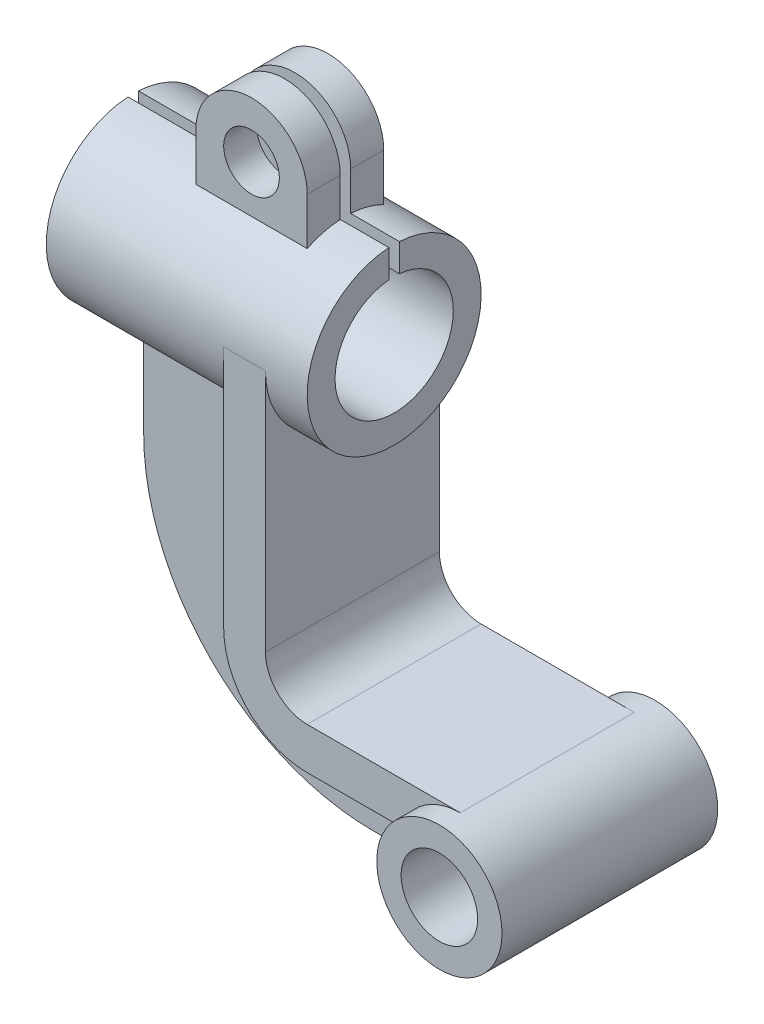
ISO-10303-21;
HEADER;
FILE_DESCRIPTION(('STEP AP214'),'2;1');
FILE_NAME('part.step','',(''),(''),'','','');
FILE_SCHEMA(('AUTOMOTIVE_DESIGN { 1 0 10303 214 1 1 1 1 }'));
ENDSEC;
DATA;
#1=APPLICATION_CONTEXT('core data for automotive mechanical design processes');
#2=APPLICATION_PROTOCOL_DEFINITION('international standard','automotive_design',2000,#1);
#3=PRODUCT_CONTEXT('',#1,'mechanical');
#4=PRODUCT('Part','Part','',(#3));
#5=PRODUCT_RELATED_PRODUCT_CATEGORY('part','',(#4));
#6=PRODUCT_DEFINITION_FORMATION('','',#4);
#7=PRODUCT_DEFINITION_CONTEXT('part definition',#1,'design');
#8=PRODUCT_DEFINITION('design','',#6,#7);
#9=PRODUCT_DEFINITION_SHAPE('','',#8);
#10=(LENGTH_UNIT() NAMED_UNIT(*) SI_UNIT(.MILLI.,.METRE.));
#11=(NAMED_UNIT(*) PLANE_ANGLE_UNIT() SI_UNIT($,.RADIAN.));
#12=(NAMED_UNIT(*) SI_UNIT($,.STERADIAN.) SOLID_ANGLE_UNIT());
#13=UNCERTAINTY_MEASURE_WITH_UNIT(LENGTH_MEASURE(1.E-05),#10,'distance_accuracy_value','');
#14=(GEOMETRIC_REPRESENTATION_CONTEXT(3) GLOBAL_UNCERTAINTY_ASSIGNED_CONTEXT((#13)) GLOBAL_UNIT_ASSIGNED_CONTEXT((#10,
#11,#12)) REPRESENTATION_CONTEXT('',''));
#15=CARTESIAN_POINT('',(0.,0.,0.));
#16=DIRECTION('',(0.,0.,1.));
#17=DIRECTION('',(1.,0.,0.));
#18=AXIS2_PLACEMENT_3D('',#15,#16,#17);
#19=CARTESIAN_POINT('',(0.,0.,25.));
#20=DIRECTION('',(0.,0.,1.));
#21=DIRECTION('',(1.,0.,0.));
#22=AXIS2_PLACEMENT_3D('',#19,#20,#21);
#23=PLANE('',#22);
#24=DIRECTION('',(-1.,0.,0.));
#25=VECTOR('',#24,1.);
#26=CARTESIAN_POINT('',(3.00056346837149E-13,-94.0000000000003,25.));
#27=LINE('',#26,#25);
#28=CARTESIAN_POINT('',(102.029437251523,-93.9999999999999,25.));
#29=VERTEX_POINT('',#28);
#30=CARTESIAN_POINT('',(75.0000000000001,-94.,25.));
#31=VERTEX_POINT('',#30);
#32=EDGE_CURVE('E951',#29,#31,#27,.T.);
#33=ORIENTED_EDGE('',*,*,#32,.F.);
#34=CARTESIAN_POINT('',(119.,-100.,25.));
#35=DIRECTION('',(0.,0.,1.));
#36=DIRECTION('',(1.,0.,0.));
#37=AXIS2_PLACEMENT_3D('',#34,#35,#36);
#38=CIRCLE('',#37,18.);
#39=CARTESIAN_POINT('',(119.,-82.,25.));
#40=VERTEX_POINT('',#39);
#41=EDGE_CURVE('E249',#29,#40,#38,.F.);
#42=ORIENTED_EDGE('',*,*,#41,.T.);
#43=DIRECTION('',(1.,0.,0.));
#44=VECTOR('',#43,1.);
#45=CARTESIAN_POINT('',(0.,-82.,25.));
#46=LINE('',#45,#44);
#47=CARTESIAN_POINT('',(75.0000000000001,-82.,25.));
#48=VERTEX_POINT('',#47);
#49=EDGE_CURVE('E277',#48,#40,#46,.T.);
#50=ORIENTED_EDGE('',*,*,#49,.F.);
#51=CARTESIAN_POINT('',(75.,-70.,25.));
#52=DIRECTION('',(0.,0.,1.));
#53=DIRECTION('',(1.,0.,0.));
#54=AXIS2_PLACEMENT_3D('',#51,#52,#53);
#55=CIRCLE('',#54,12.);
#56=CARTESIAN_POINT('',(63.,-69.9999999999999,25.));
#57=VERTEX_POINT('',#56);
#58=EDGE_CURVE('E268',#57,#48,#55,.T.);
#59=ORIENTED_EDGE('',*,*,#58,.F.);
#60=DIRECTION('',(0.,-1.,0.));
#61=VECTOR('',#60,1.);
#62=CARTESIAN_POINT('',(63.,0.,25.));
#63=LINE('',#62,#61);
#64=CARTESIAN_POINT('',(63.,0.,25.));
#65=VERTEX_POINT('',#64);
#66=EDGE_CURVE('E945',#65,#57,#63,.T.);
#67=ORIENTED_EDGE('',*,*,#66,.F.);
#68=DIRECTION('',(1.,0.,0.));
#69=VECTOR('',#68,1.);
#70=CARTESIAN_POINT('',(0.,0.,25.));
#71=LINE('',#70,#69);
#72=CARTESIAN_POINT('',(51.,0.,25.));
#73=VERTEX_POINT('',#72);
#74=EDGE_CURVE('E944',#73,#65,#71,.T.);
#75=ORIENTED_EDGE('',*,*,#74,.F.);
#76=DIRECTION('',(0.,1.,0.));
#77=VECTOR('',#76,1.);
#78=CARTESIAN_POINT('',(51.,0.,25.));
#79=LINE('',#78,#77);
#80=CARTESIAN_POINT('',(51.,-69.9999999999999,25.));
#81=VERTEX_POINT('',#80);
#82=EDGE_CURVE('E949',#81,#73,#79,.T.);
#83=ORIENTED_EDGE('',*,*,#82,.F.);
#84=CARTESIAN_POINT('',(75.,-70.,25.));
#85=DIRECTION('',(0.,0.,1.));
#86=DIRECTION('',(1.,0.,0.));
#87=AXIS2_PLACEMENT_3D('',#84,#85,#86);
#88=CIRCLE('',#87,24.);
#89=EDGE_CURVE('E952',#81,#31,#88,.T.);
#90=ORIENTED_EDGE('',*,*,#89,.T.);
#91=EDGE_LOOP('',(#33,#42,#50,#59,#67,#75,#83,#90));
#92=FACE_BOUND('',#91,.T.);
#93=ADVANCED_FACE('F52',(#92),#23,.T.);
#94=CARTESIAN_POINT('',(0.,0.,-25.));
#95=DIRECTION('',(0.,0.,1.));
#96=DIRECTION('',(1.,0.,0.));
#97=AXIS2_PLACEMENT_3D('',#94,#95,#96);
#98=PLANE('',#97);
#99=CARTESIAN_POINT('',(119.,-100.,-25.));
#100=DIRECTION('',(0.,0.,1.));
#101=DIRECTION('',(1.,0.,0.));
#102=AXIS2_PLACEMENT_3D('',#99,#100,#101);
#103=CIRCLE('',#102,18.);
#104=CARTESIAN_POINT('',(102.029437251523,-93.9999999999999,-25.));
#105=VERTEX_POINT('',#104);
#106=CARTESIAN_POINT('',(119.,-82.,-25.));
#107=VERTEX_POINT('',#106);
#108=EDGE_CURVE('E237',#105,#107,#103,.F.);
#109=ORIENTED_EDGE('',*,*,#108,.F.);
#110=DIRECTION('',(-1.,0.,0.));
#111=VECTOR('',#110,1.);
#112=CARTESIAN_POINT('',(3.00056346837149E-13,-94.0000000000003,-25.));
#113=LINE('',#112,#111);
#114=CARTESIAN_POINT('',(75.0000000000001,-94.,-25.));
#115=VERTEX_POINT('',#114);
#116=EDGE_CURVE('E243',#105,#115,#113,.T.);
#117=ORIENTED_EDGE('',*,*,#116,.T.);
#118=CARTESIAN_POINT('',(75.,-70.,-25.));
#119=DIRECTION('',(0.,0.,1.));
#120=DIRECTION('',(1.,0.,0.));
#121=AXIS2_PLACEMENT_3D('',#118,#119,#120);
#122=CIRCLE('',#121,24.);
#123=CARTESIAN_POINT('',(51.,-69.9999999999999,-25.));
#124=VERTEX_POINT('',#123);
#125=EDGE_CURVE('E266',#124,#115,#122,.T.);
#126=ORIENTED_EDGE('',*,*,#125,.F.);
#127=DIRECTION('',(0.,1.,0.));
#128=VECTOR('',#127,1.);
#129=CARTESIAN_POINT('',(51.,0.,-25.));
#130=LINE('',#129,#128);
#131=CARTESIAN_POINT('',(51.,0.,-25.));
#132=VERTEX_POINT('',#131);
#133=EDGE_CURVE('E269',#124,#132,#130,.T.);
#134=ORIENTED_EDGE('',*,*,#133,.T.);
#135=DIRECTION('',(1.,0.,0.));
#136=VECTOR('',#135,1.);
#137=CARTESIAN_POINT('',(0.,0.,-25.));
#138=LINE('',#137,#136);
#139=CARTESIAN_POINT('',(63.,0.,-25.));
#140=VERTEX_POINT('',#139);
#141=EDGE_CURVE('E962',#132,#140,#138,.T.);
#142=ORIENTED_EDGE('',*,*,#141,.T.);
#143=DIRECTION('',(0.,-1.,0.));
#144=VECTOR('',#143,1.);
#145=CARTESIAN_POINT('',(63.,0.,-25.));
#146=LINE('',#145,#144);
#147=CARTESIAN_POINT('',(63.,-69.9999999999999,-25.));
#148=VERTEX_POINT('',#147);
#149=EDGE_CURVE('E956',#140,#148,#146,.T.);
#150=ORIENTED_EDGE('',*,*,#149,.T.);
#151=CARTESIAN_POINT('',(75.,-70.,-25.));
#152=DIRECTION('',(0.,0.,1.));
#153=DIRECTION('',(1.,0.,0.));
#154=AXIS2_PLACEMENT_3D('',#151,#152,#153);
#155=CIRCLE('',#154,12.);
#156=CARTESIAN_POINT('',(75.0000000000001,-82.,-25.));
#157=VERTEX_POINT('',#156);
#158=EDGE_CURVE('E936',#148,#157,#155,.T.);
#159=ORIENTED_EDGE('',*,*,#158,.T.);
#160=DIRECTION('',(1.,0.,0.));
#161=VECTOR('',#160,1.);
#162=CARTESIAN_POINT('',(0.,-82.,-25.));
#163=LINE('',#162,#161);
#164=EDGE_CURVE('E242',#157,#107,#163,.T.);
#165=ORIENTED_EDGE('',*,*,#164,.T.);
#166=EDGE_LOOP('',(#109,#117,#126,#134,#142,#150,#159,#165));
#167=FACE_BOUND('',#166,.T.);
#168=ADVANCED_FACE('F236',(#167),#98,.F.);
#169=CARTESIAN_POINT('',(51.,0.,25.));
#170=DIRECTION('',(-1.,0.,0.));
#171=DIRECTION('',(0.,0.,1.));
#172=AXIS2_PLACEMENT_3D('',#169,#170,#171);
#173=PLANE('',#172);
#174=DIRECTION('',(0.,0.,-1.));
#175=VECTOR('',#174,1.);
#176=CARTESIAN_POINT('',(51.,-69.9999999999999,25.));
#177=LINE('',#176,#175);
#178=CARTESIAN_POINT('',(51.,-69.9999999999999,-6.));
#179=VERTEX_POINT('',#178);
#180=EDGE_CURVE('E285',#179,#124,#177,.T.);
#181=ORIENTED_EDGE('',*,*,#180,.F.);
#182=DIRECTION('',(0.,1.,0.));
#183=VECTOR('',#182,1.);
#184=CARTESIAN_POINT('',(51.,0.,-6.));
#185=LINE('',#184,#183);
#186=CARTESIAN_POINT('',(51.,-24.2693221990232,-6.));
#187=VERTEX_POINT('',#186);
#188=EDGE_CURVE('E918',#179,#187,#185,.T.);
#189=ORIENTED_EDGE('',*,*,#188,.T.);
#190=CARTESIAN_POINT('',(51.,0.,0.));
#191=DIRECTION('',(-1.,0.,0.));
#192=DIRECTION('',(0.,0.,1.));
#193=AXIS2_PLACEMENT_3D('',#190,#191,#192);
#194=CIRCLE('',#193,25.);
#195=EDGE_CURVE('E286',#132,#187,#194,.T.);
#196=ORIENTED_EDGE('',*,*,#195,.F.);
#197=ORIENTED_EDGE('',*,*,#133,.F.);
#198=EDGE_LOOP('',(#181,#189,#196,#197));
#199=FACE_BOUND('',#198,.T.);
#200=ADVANCED_FACE('F456',(#199),#173,.T.);
#201=CARTESIAN_POINT('',(75.,-70.,25.));
#202=DIRECTION('',(0.,0.,-1.));
#203=DIRECTION('',(-1.,0.,0.));
#204=AXIS2_PLACEMENT_3D('',#201,#202,#203);
#205=CYLINDRICAL_SURFACE('',#204,24.);
#206=CARTESIAN_POINT('',(75.,-70.,-6.));
#207=DIRECTION('',(0.,0.,1.));
#208=DIRECTION('',(1.,0.,0.));
#209=AXIS2_PLACEMENT_3D('',#206,#207,#208);
#210=CIRCLE('',#209,24.);
#211=CARTESIAN_POINT('',(75.0000000000001,-94.,-6.));
#212=VERTEX_POINT('',#211);
#213=EDGE_CURVE('E911',#179,#212,#210,.T.);
#214=ORIENTED_EDGE('',*,*,#213,.F.);
#215=ORIENTED_EDGE('',*,*,#180,.T.);
#216=ORIENTED_EDGE('',*,*,#125,.T.);
#217=DIRECTION('',(0.,0.,-1.));
#218=VECTOR('',#217,1.);
#219=CARTESIAN_POINT('',(75.0000000000001,-94.,25.));
#220=LINE('',#219,#218);
#221=EDGE_CURVE('E262',#212,#115,#220,.T.);
#222=ORIENTED_EDGE('',*,*,#221,.F.);
#223=EDGE_LOOP('',(#214,#215,#216,#222));
#224=FACE_BOUND('',#223,.T.);
#225=ADVANCED_FACE('F486',(#224),#205,.T.);
#226=CARTESIAN_POINT('',(3.00056346837149E-13,-94.0000000000003,25.));
#227=DIRECTION('',(0.,-1.,0.));
#228=DIRECTION('',(1.,0.,0.));
#229=AXIS2_PLACEMENT_3D('',#226,#227,#228);
#230=PLANE('',#229);
#231=DIRECTION('',(0.,0.,-1.));
#232=VECTOR('',#231,1.);
#233=CARTESIAN_POINT('',(102.029437251523,-93.9999999999999,25.));
#234=LINE('',#233,#232);
#235=CARTESIAN_POINT('',(102.029437251523,-93.9999999999999,-6.));
#236=VERTEX_POINT('',#235);
#237=EDGE_CURVE('E252',#236,#105,#234,.T.);
#238=ORIENTED_EDGE('',*,*,#237,.F.);
#239=DIRECTION('',(-1.,0.,0.));
#240=VECTOR('',#239,1.);
#241=CARTESIAN_POINT('',(3.00056346837149E-13,-94.0000000000003,-6.));
#242=LINE('',#241,#240);
#243=EDGE_CURVE('E920',#236,#212,#242,.T.);
#244=ORIENTED_EDGE('',*,*,#243,.T.);
#245=ORIENTED_EDGE('',*,*,#221,.T.);
#246=ORIENTED_EDGE('',*,*,#116,.F.);
#247=EDGE_LOOP('',(#238,#244,#245,#246));
#248=FACE_BOUND('',#247,.T.);
#249=ADVANCED_FACE('F265',(#248),#230,.T.);
#250=CARTESIAN_POINT('',(75.,0.,0.));
#251=DIRECTION('',(-1.,0.,0.));
#252=DIRECTION('',(0.,0.,1.));
#253=AXIS2_PLACEMENT_3D('',#250,#251,#252);
#254=CYLINDRICAL_SURFACE('',#253,25.);
#255=DIRECTION('',(-1.,0.,0.));
#256=VECTOR('',#255,1.);
#257=CARTESIAN_POINT('',(75.,24.9549594269356,1.5));
#258=LINE('',#257,#256);
#259=CARTESIAN_POINT('',(29.,24.9549594269356,1.5));
#260=VERTEX_POINT('',#259);
#261=CARTESIAN_POINT('',(0.,24.9549594269356,1.5));
#262=VERTEX_POINT('',#261);
#263=EDGE_CURVE('E365',#260,#262,#258,.T.);
#264=ORIENTED_EDGE('',*,*,#263,.T.);
#265=CARTESIAN_POINT('',(0.,0.,0.));
#266=DIRECTION('',(1.,0.,0.));
#267=DIRECTION('',(0.,0.,-1.));
#268=AXIS2_PLACEMENT_3D('',#265,#266,#267);
#269=CIRCLE('',#268,25.);
#270=CARTESIAN_POINT('',(0.,24.9549594269356,-1.5));
#271=VERTEX_POINT('',#270);
#272=EDGE_CURVE('E352',#262,#271,#269,.T.);
#273=ORIENTED_EDGE('',*,*,#272,.T.);
#274=DIRECTION('',(-1.,0.,0.));
#275=VECTOR('',#274,1.);
#276=CARTESIAN_POINT('',(75.,24.9549594269356,-1.5));
#277=LINE('',#276,#275);
#278=CARTESIAN_POINT('',(29.,24.9549594269356,-1.5));
#279=VERTEX_POINT('',#278);
#280=EDGE_CURVE('E385',#279,#271,#277,.T.);
#281=ORIENTED_EDGE('',*,*,#280,.F.);
#282=CARTESIAN_POINT('',(29.,0.,0.));
#283=DIRECTION('',(-1.,0.,0.));
#284=DIRECTION('',(0.,0.,1.));
#285=AXIS2_PLACEMENT_3D('',#282,#283,#284);
#286=CIRCLE('',#285,25.);
#287=CARTESIAN_POINT('',(29.,22.4499443206436,-11.));
#288=VERTEX_POINT('',#287);
#289=EDGE_CURVE('E349',#279,#288,#286,.T.);
#290=ORIENTED_EDGE('',*,*,#289,.T.);
#291=DIRECTION('',(-1.,0.,0.));
#292=VECTOR('',#291,1.);
#293=CARTESIAN_POINT('',(75.,22.4499443206436,-11.));
#294=LINE('',#293,#292);
#295=CARTESIAN_POINT('',(61.,22.4499443206436,-11.));
#296=VERTEX_POINT('',#295);
#297=EDGE_CURVE('E387',#296,#288,#294,.T.);
#298=ORIENTED_EDGE('',*,*,#297,.F.);
#299=CARTESIAN_POINT('',(61.,0.,0.));
#300=DIRECTION('',(1.,0.,0.));
#301=DIRECTION('',(0.,0.,-1.));
#302=AXIS2_PLACEMENT_3D('',#299,#300,#301);
#303=CIRCLE('',#302,25.);
#304=CARTESIAN_POINT('',(61.,24.9549594269356,-1.5));
#305=VERTEX_POINT('',#304);
#306=EDGE_CURVE('E355',#296,#305,#303,.T.);
#307=ORIENTED_EDGE('',*,*,#306,.T.);
#308=CARTESIAN_POINT('',(75.,24.9549594269356,-1.5));
#309=VERTEX_POINT('',#308);
#310=EDGE_CURVE('E382',#309,#305,#277,.T.);
#311=ORIENTED_EDGE('',*,*,#310,.F.);
#312=CARTESIAN_POINT('',(75.,0.,0.));
#313=DIRECTION('',(1.,0.,0.));
#314=DIRECTION('',(0.,0.,-1.));
#315=AXIS2_PLACEMENT_3D('',#312,#313,#314);
#316=CIRCLE('',#315,25.);
#317=CARTESIAN_POINT('',(75.,24.9549594269356,1.5));
#318=VERTEX_POINT('',#317);
#319=EDGE_CURVE('E354',#318,#309,#316,.T.);
#320=ORIENTED_EDGE('',*,*,#319,.F.);
#321=CARTESIAN_POINT('',(61.,24.9549594269356,1.5));
#322=VERTEX_POINT('',#321);
#323=EDGE_CURVE('E374',#318,#322,#258,.T.);
#324=ORIENTED_EDGE('',*,*,#323,.T.);
#325=CARTESIAN_POINT('',(61.,0.,0.));
#326=DIRECTION('',(1.,0.,0.));
#327=DIRECTION('',(0.,0.,-1.));
#328=AXIS2_PLACEMENT_3D('',#325,#326,#327);
#329=CIRCLE('',#328,25.);
#330=CARTESIAN_POINT('',(61.,22.4499443206436,11.));
#331=VERTEX_POINT('',#330);
#332=EDGE_CURVE('E325',#322,#331,#329,.T.);
#333=ORIENTED_EDGE('',*,*,#332,.T.);
#334=DIRECTION('',(-1.,0.,0.));
#335=VECTOR('',#334,1.);
#336=CARTESIAN_POINT('',(75.,22.4499443206436,11.));
#337=LINE('',#336,#335);
#338=CARTESIAN_POINT('',(29.,22.4499443206436,11.));
#339=VERTEX_POINT('',#338);
#340=EDGE_CURVE('E63',#331,#339,#337,.T.);
#341=ORIENTED_EDGE('',*,*,#340,.T.);
#342=CARTESIAN_POINT('',(29.,0.,0.));
#343=DIRECTION('',(-1.,0.,0.));
#344=DIRECTION('',(0.,0.,1.));
#345=AXIS2_PLACEMENT_3D('',#342,#343,#344);
#346=CIRCLE('',#345,25.);
#347=EDGE_CURVE('E317',#339,#260,#346,.T.);
#348=ORIENTED_EDGE('',*,*,#347,.T.);
#349=EDGE_LOOP('',(#264,#273,#281,#290,#298,#307,#311,#320,#324,#333,#341,#348));
#350=FACE_BOUND('',#349,.T.);
#351=CARTESIAN_POINT('',(63.,0.,0.));
#352=DIRECTION('',(1.,0.,0.));
#353=DIRECTION('',(0.,1.,0.));
#354=AXIS2_PLACEMENT_3D('',#351,#352,#353);
#355=CIRCLE('',#354,25.);
#356=EDGE_CURVE('E292',#65,#140,#355,.T.);
#357=ORIENTED_EDGE('',*,*,#356,.T.);
#358=ORIENTED_EDGE('',*,*,#141,.F.);
#359=ORIENTED_EDGE('',*,*,#195,.T.);
#360=DIRECTION('',(-1.,0.,0.));
#361=VECTOR('',#360,1.);
#362=CARTESIAN_POINT('',(75.,-24.2693221990232,-6.));
#363=LINE('',#362,#361);
#364=CARTESIAN_POINT('',(8.99999999999999,-24.2693221990232,-6.));
#365=VERTEX_POINT('',#364);
#366=EDGE_CURVE('E71',#365,#187,#363,.F.);
#367=ORIENTED_EDGE('',*,*,#366,.F.);
#368=CARTESIAN_POINT('',(8.99999999999999,0.,0.));
#369=DIRECTION('',(-1.,0.,0.));
#370=DIRECTION('',(0.,0.,1.));
#371=AXIS2_PLACEMENT_3D('',#368,#369,#370);
#372=CIRCLE('',#371,25.);
#373=CARTESIAN_POINT('',(8.99999999999999,-24.2693221990232,6.));
#374=VERTEX_POINT('',#373);
#375=EDGE_CURVE('E69',#365,#374,#372,.T.);
#376=ORIENTED_EDGE('',*,*,#375,.T.);
#377=DIRECTION('',(-1.,0.,0.));
#378=VECTOR('',#377,1.);
#379=CARTESIAN_POINT('',(75.,-24.2693221990232,6.));
#380=LINE('',#379,#378);
#381=CARTESIAN_POINT('',(51.,-24.2693221990232,6.));
#382=VERTEX_POINT('',#381);
#383=EDGE_CURVE('E927',#374,#382,#380,.F.);
#384=ORIENTED_EDGE('',*,*,#383,.T.);
#385=EDGE_CURVE('E289',#382,#73,#194,.T.);
#386=ORIENTED_EDGE('',*,*,#385,.T.);
#387=ORIENTED_EDGE('',*,*,#74,.T.);
#388=EDGE_LOOP('',(#357,#358,#359,#367,#376,#384,#386,#387));
#389=FACE_BOUND('',#388,.T.);
#390=ADVANCED_FACE('F54',(#350,#389),#254,.T.);
#391=CARTESIAN_POINT('',(75.,16.9336942218761,-1.5));
#392=DIRECTION('',(0.,0.,-1.));
#393=DIRECTION('',(-1.,0.,0.));
#394=AXIS2_PLACEMENT_3D('',#391,#392,#393);
#395=PLANE('',#394);
#396=DIRECTION('',(0.,-1.,0.));
#397=VECTOR('',#396,1.);
#398=CARTESIAN_POINT('',(0.,16.9336942218761,-1.5));
#399=LINE('',#398,#397);
#400=CARTESIAN_POINT('',(0.,16.9336942218761,-1.5));
#401=VERTEX_POINT('',#400);
#402=EDGE_CURVE('E370',#271,#401,#399,.T.);
#403=ORIENTED_EDGE('',*,*,#402,.T.);
#404=DIRECTION('',(-1.,0.,0.));
#405=VECTOR('',#404,1.);
#406=CARTESIAN_POINT('',(75.,16.9336942218761,-1.5));
#407=LINE('',#406,#405);
#408=CARTESIAN_POINT('',(75.,16.9336942218761,-1.5));
#409=VERTEX_POINT('',#408);
#410=EDGE_CURVE('E379',#409,#401,#407,.T.);
#411=ORIENTED_EDGE('',*,*,#410,.F.);
#412=DIRECTION('',(0.,-1.,0.));
#413=VECTOR('',#412,1.);
#414=CARTESIAN_POINT('',(75.,16.9336942218761,-1.5));
#415=LINE('',#414,#413);
#416=EDGE_CURVE('E360',#309,#409,#415,.T.);
#417=ORIENTED_EDGE('',*,*,#416,.F.);
#418=ORIENTED_EDGE('',*,*,#310,.T.);
#419=DIRECTION('',(0.,1.,0.));
#420=VECTOR('',#419,1.);
#421=CARTESIAN_POINT('',(61.,20.,-1.5));
#422=LINE('',#421,#420);
#423=CARTESIAN_POINT('',(61.,36.,-1.5));
#424=VERTEX_POINT('',#423);
#425=EDGE_CURVE('E333',#305,#424,#422,.T.);
#426=ORIENTED_EDGE('',*,*,#425,.T.);
#427=CARTESIAN_POINT('',(45.,36.,-1.5));
#428=DIRECTION('',(0.,0.,1.));
#429=DIRECTION('',(1.,0.,0.));
#430=AXIS2_PLACEMENT_3D('',#427,#428,#429);
#431=CIRCLE('',#430,16.);
#432=CARTESIAN_POINT('',(29.,36.,-1.5));
#433=VERTEX_POINT('',#432);
#434=EDGE_CURVE('E327',#424,#433,#431,.T.);
#435=ORIENTED_EDGE('',*,*,#434,.T.);
#436=DIRECTION('',(0.,-1.,0.));
#437=VECTOR('',#436,1.);
#438=CARTESIAN_POINT('',(29.,36.,-1.5));
#439=LINE('',#438,#437);
#440=EDGE_CURVE('E344',#433,#279,#439,.T.);
#441=ORIENTED_EDGE('',*,*,#440,.T.);
#442=ORIENTED_EDGE('',*,*,#280,.T.);
#443=EDGE_LOOP('',(#403,#411,#417,#418,#426,#435,#441,#442));
#444=FACE_BOUND('',#443,.T.);
#445=CARTESIAN_POINT('',(45.,36.,-1.5));
#446=DIRECTION('',(0.,0.,1.));
#447=DIRECTION('',(1.,0.,0.));
#448=AXIS2_PLACEMENT_3D('',#445,#446,#447);
#449=CIRCLE('',#448,8.);
#450=CARTESIAN_POINT('',(53.,36.,-1.5));
#451=VERTEX_POINT('',#450);
#452=EDGE_CURVE('E322',#451,#451,#449,.T.);
#453=ORIENTED_EDGE('',*,*,#452,.F.);
#454=EDGE_LOOP('',(#453));
#455=FACE_BOUND('',#454,.T.);
#456=ADVANCED_FACE('F420',(#444,#455),#395,.F.);
#457=CARTESIAN_POINT('',(75.,0.,0.));
#458=DIRECTION('',(-1.,0.,0.));
#459=DIRECTION('',(0.,0.,1.));
#460=AXIS2_PLACEMENT_3D('',#457,#458,#459);
#461=CYLINDRICAL_SURFACE('',#460,17.);
#462=ORIENTED_EDGE('',*,*,#410,.T.);
#463=CARTESIAN_POINT('',(0.,0.,0.));
#464=DIRECTION('',(-1.,0.,0.));
#465=DIRECTION('',(0.,0.,-1.));
#466=AXIS2_PLACEMENT_3D('',#463,#464,#465);
#467=CIRCLE('',#466,17.);
#468=CARTESIAN_POINT('',(0.,16.9336942218761,1.5));
#469=VERTEX_POINT('',#468);
#470=EDGE_CURVE('E367',#401,#469,#467,.T.);
#471=ORIENTED_EDGE('',*,*,#470,.T.);
#472=DIRECTION('',(-1.,0.,0.));
#473=VECTOR('',#472,1.);
#474=CARTESIAN_POINT('',(75.,16.9336942218761,1.5));
#475=LINE('',#474,#473);
#476=CARTESIAN_POINT('',(75.,16.9336942218761,1.5));
#477=VERTEX_POINT('',#476);
#478=EDGE_CURVE('E378',#477,#469,#475,.T.);
#479=ORIENTED_EDGE('',*,*,#478,.F.);
#480=CARTESIAN_POINT('',(75.,0.,0.));
#481=DIRECTION('',(-1.,0.,0.));
#482=DIRECTION('',(0.,0.,-1.));
#483=AXIS2_PLACEMENT_3D('',#480,#481,#482);
#484=CIRCLE('',#483,17.);
#485=EDGE_CURVE('E358',#409,#477,#484,.T.);
#486=ORIENTED_EDGE('',*,*,#485,.F.);
#487=EDGE_LOOP('',(#462,#471,#479,#486));
#488=FACE_BOUND('',#487,.T.);
#489=ADVANCED_FACE('F823',(#488),#461,.F.);
#490=CARTESIAN_POINT('',(75.,16.9336942218761,1.5));
#491=DIRECTION('',(0.,0.,1.));
#492=DIRECTION('',(1.,0.,0.));
#493=AXIS2_PLACEMENT_3D('',#490,#491,#492);
#494=PLANE('',#493);
#495=DIRECTION('',(0.,1.,0.));
#496=VECTOR('',#495,1.);
#497=CARTESIAN_POINT('',(0.,16.9336942218761,1.5));
#498=LINE('',#497,#496);
#499=EDGE_CURVE('E359',#469,#262,#498,.T.);
#500=ORIENTED_EDGE('',*,*,#499,.T.);
#501=ORIENTED_EDGE('',*,*,#263,.F.);
#502=DIRECTION('',(0.,1.,0.));
#503=VECTOR('',#502,1.);
#504=CARTESIAN_POINT('',(29.,16.9336942218761,1.5));
#505=LINE('',#504,#503);
#506=CARTESIAN_POINT('',(29.,36.,1.5));
#507=VERTEX_POINT('',#506);
#508=EDGE_CURVE('E315',#260,#507,#505,.T.);
#509=ORIENTED_EDGE('',*,*,#508,.T.);
#510=CARTESIAN_POINT('',(45.,36.,1.5));
#511=DIRECTION('',(0.,0.,1.));
#512=DIRECTION('',(1.,0.,0.));
#513=AXIS2_PLACEMENT_3D('',#510,#511,#512);
#514=CIRCLE('',#513,16.);
#515=CARTESIAN_POINT('',(61.,36.,1.5));
#516=VERTEX_POINT('',#515);
#517=EDGE_CURVE('E301',#516,#507,#514,.T.);
#518=ORIENTED_EDGE('',*,*,#517,.F.);
#519=DIRECTION('',(0.,-1.,0.));
#520=VECTOR('',#519,1.);
#521=CARTESIAN_POINT('',(61.,16.9336942218761,1.5));
#522=LINE('',#521,#520);
#523=EDGE_CURVE('E300',#516,#322,#522,.T.);
#524=ORIENTED_EDGE('',*,*,#523,.T.);
#525=ORIENTED_EDGE('',*,*,#323,.F.);
#526=DIRECTION('',(0.,1.,0.));
#527=VECTOR('',#526,1.);
#528=CARTESIAN_POINT('',(75.,16.9336942218761,1.5));
#529=LINE('',#528,#527);
#530=EDGE_CURVE('E362',#477,#318,#529,.T.);
#531=ORIENTED_EDGE('',*,*,#530,.F.);
#532=ORIENTED_EDGE('',*,*,#478,.T.);
#533=EDGE_LOOP('',(#500,#501,#509,#518,#524,#525,#531,#532));
#534=FACE_BOUND('',#533,.T.);
#535=CARTESIAN_POINT('',(45.,36.,1.5));
#536=DIRECTION('',(0.,0.,1.));
#537=DIRECTION('',(1.,0.,0.));
#538=AXIS2_PLACEMENT_3D('',#535,#536,#537);
#539=CIRCLE('',#538,8.);
#540=CARTESIAN_POINT('',(53.,36.,1.5));
#541=VERTEX_POINT('',#540);
#542=EDGE_CURVE('E291',#541,#541,#539,.T.);
#543=ORIENTED_EDGE('',*,*,#542,.T.);
#544=EDGE_LOOP('',(#543));
#545=FACE_BOUND('',#544,.T.);
#546=ADVANCED_FACE('F406',(#534,#545),#494,.F.);
#547=CARTESIAN_POINT('',(75.,0.,0.));
#548=DIRECTION('',(1.,0.,0.));
#549=DIRECTION('',(0.,0.,-1.));
#550=AXIS2_PLACEMENT_3D('',#547,#548,#549);
#551=PLANE('',#550);
#552=ORIENTED_EDGE('',*,*,#485,.T.);
#553=ORIENTED_EDGE('',*,*,#530,.T.);
#554=ORIENTED_EDGE('',*,*,#319,.T.);
#555=ORIENTED_EDGE('',*,*,#416,.T.);
#556=EDGE_LOOP('',(#552,#553,#554,#555));
#557=FACE_BOUND('',#556,.T.);
#558=ADVANCED_FACE('F807',(#557),#551,.T.);
#559=CARTESIAN_POINT('',(0.,0.,0.));
#560=DIRECTION('',(1.,0.,0.));
#561=DIRECTION('',(0.,0.,-1.));
#562=AXIS2_PLACEMENT_3D('',#559,#560,#561);
#563=PLANE('',#562);
#564=ORIENTED_EDGE('',*,*,#272,.F.);
#565=ORIENTED_EDGE('',*,*,#499,.F.);
#566=ORIENTED_EDGE('',*,*,#470,.F.);
#567=ORIENTED_EDGE('',*,*,#402,.F.);
#568=EDGE_LOOP('',(#564,#565,#566,#567));
#569=FACE_BOUND('',#568,.T.);
#570=ADVANCED_FACE('F413',(#569),#563,.F.);
#571=CARTESIAN_POINT('',(45.,36.,-11.));
#572=DIRECTION('',(0.,0.,1.));
#573=DIRECTION('',(1.,0.,0.));
#574=AXIS2_PLACEMENT_3D('',#571,#572,#573);
#575=PLANE('',#574);
#576=CARTESIAN_POINT('',(45.,36.,-11.));
#577=DIRECTION('',(0.,0.,1.));
#578=DIRECTION('',(1.,0.,0.));
#579=AXIS2_PLACEMENT_3D('',#576,#577,#578);
#580=CIRCLE('',#579,8.);
#581=CARTESIAN_POINT('',(53.,36.,-11.));
#582=VERTEX_POINT('',#581);
#583=EDGE_CURVE('E324',#582,#582,#580,.T.);
#584=ORIENTED_EDGE('',*,*,#583,.T.);
#585=EDGE_LOOP('',(#584));
#586=FACE_BOUND('',#585,.T.);
#587=DIRECTION('',(0.,1.,0.));
#588=VECTOR('',#587,1.);
#589=CARTESIAN_POINT('',(61.,20.,-11.));
#590=LINE('',#589,#588);
#591=CARTESIAN_POINT('',(61.,36.,-11.));
#592=VERTEX_POINT('',#591);
#593=EDGE_CURVE('E336',#296,#592,#590,.T.);
#594=ORIENTED_EDGE('',*,*,#593,.F.);
#595=ORIENTED_EDGE('',*,*,#297,.T.);
#596=DIRECTION('',(0.,-1.,0.));
#597=VECTOR('',#596,1.);
#598=CARTESIAN_POINT('',(29.,36.,-11.));
#599=LINE('',#598,#597);
#600=CARTESIAN_POINT('',(29.,36.,-11.));
#601=VERTEX_POINT('',#600);
#602=EDGE_CURVE('E331',#601,#288,#599,.T.);
#603=ORIENTED_EDGE('',*,*,#602,.F.);
#604=CARTESIAN_POINT('',(45.,36.,-11.));
#605=DIRECTION('',(0.,0.,1.));
#606=DIRECTION('',(1.,0.,0.));
#607=AXIS2_PLACEMENT_3D('',#604,#605,#606);
#608=CIRCLE('',#607,16.);
#609=EDGE_CURVE('E332',#592,#601,#608,.T.);
#610=ORIENTED_EDGE('',*,*,#609,.F.);
#611=EDGE_LOOP('',(#594,#595,#603,#610));
#612=FACE_BOUND('',#611,.T.);
#613=ADVANCED_FACE('F435',(#586,#612),#575,.F.);
#614=CARTESIAN_POINT('',(61.,20.,-11.));
#615=DIRECTION('',(1.,0.,0.));
#616=DIRECTION('',(0.,0.,-1.));
#617=AXIS2_PLACEMENT_3D('',#614,#615,#616);
#618=PLANE('',#617);
#619=ORIENTED_EDGE('',*,*,#425,.F.);
#620=ORIENTED_EDGE('',*,*,#306,.F.);
#621=ORIENTED_EDGE('',*,*,#593,.T.);
#622=DIRECTION('',(0.,0.,1.));
#623=VECTOR('',#622,1.);
#624=CARTESIAN_POINT('',(61.,36.,-11.));
#625=LINE('',#624,#623);
#626=EDGE_CURVE('E350',#592,#424,#625,.T.);
#627=ORIENTED_EDGE('',*,*,#626,.T.);
#628=EDGE_LOOP('',(#619,#620,#621,#627));
#629=FACE_BOUND('',#628,.T.);
#630=ADVANCED_FACE('F440',(#629),#618,.T.);
#631=CARTESIAN_POINT('',(29.,36.,-11.));
#632=DIRECTION('',(-1.,0.,0.));
#633=DIRECTION('',(0.,0.,1.));
#634=AXIS2_PLACEMENT_3D('',#631,#632,#633);
#635=PLANE('',#634);
#636=ORIENTED_EDGE('',*,*,#440,.F.);
#637=DIRECTION('',(0.,0.,1.));
#638=VECTOR('',#637,1.);
#639=CARTESIAN_POINT('',(29.,36.,-11.));
#640=LINE('',#639,#638);
#641=EDGE_CURVE('E339',#601,#433,#640,.T.);
#642=ORIENTED_EDGE('',*,*,#641,.F.);
#643=ORIENTED_EDGE('',*,*,#602,.T.);
#644=ORIENTED_EDGE('',*,*,#289,.F.);
#645=EDGE_LOOP('',(#636,#642,#643,#644));
#646=FACE_BOUND('',#645,.T.);
#647=ADVANCED_FACE('F430',(#646),#635,.T.);
#648=CARTESIAN_POINT('',(45.,36.,-11.));
#649=DIRECTION('',(0.,0.,1.));
#650=DIRECTION('',(1.,0.,0.));
#651=AXIS2_PLACEMENT_3D('',#648,#649,#650);
#652=CYLINDRICAL_SURFACE('',#651,16.);
#653=ORIENTED_EDGE('',*,*,#434,.F.);
#654=ORIENTED_EDGE('',*,*,#626,.F.);
#655=ORIENTED_EDGE('',*,*,#609,.T.);
#656=ORIENTED_EDGE('',*,*,#641,.T.);
#657=EDGE_LOOP('',(#653,#654,#655,#656));
#658=FACE_BOUND('',#657,.T.);
#659=ADVANCED_FACE('F438',(#658),#652,.T.);
#660=CARTESIAN_POINT('',(45.,36.,-11.));
#661=DIRECTION('',(0.,0.,1.));
#662=DIRECTION('',(1.,0.,0.));
#663=AXIS2_PLACEMENT_3D('',#660,#661,#662);
#664=CYLINDRICAL_SURFACE('',#663,8.);
#665=ORIENTED_EDGE('',*,*,#452,.T.);
#666=EDGE_LOOP('',(#665));
#667=FACE_BOUND('',#666,.T.);
#668=ORIENTED_EDGE('',*,*,#583,.F.);
#669=EDGE_LOOP('',(#668));
#670=FACE_BOUND('',#669,.T.);
#671=ADVANCED_FACE('F442',(#667,#670),#664,.F.);
#672=CARTESIAN_POINT('',(45.,36.,11.));
#673=DIRECTION('',(0.,0.,1.));
#674=DIRECTION('',(1.,0.,0.));
#675=AXIS2_PLACEMENT_3D('',#672,#673,#674);
#676=PLANE('',#675);
#677=CARTESIAN_POINT('',(45.,36.,11.));
#678=DIRECTION('',(0.,0.,1.));
#679=DIRECTION('',(1.,0.,0.));
#680=AXIS2_PLACEMENT_3D('',#677,#678,#679);
#681=CIRCLE('',#680,8.);
#682=CARTESIAN_POINT('',(53.,36.,11.));
#683=VERTEX_POINT('',#682);
#684=EDGE_CURVE('E294',#683,#683,#681,.T.);
#685=ORIENTED_EDGE('',*,*,#684,.F.);
#686=EDGE_LOOP('',(#685));
#687=FACE_BOUND('',#686,.T.);
#688=ORIENTED_EDGE('',*,*,#340,.F.);
#689=DIRECTION('',(0.,-1.,0.));
#690=VECTOR('',#689,1.);
#691=CARTESIAN_POINT('',(61.,16.9336942218761,11.));
#692=LINE('',#691,#690);
#693=CARTESIAN_POINT('',(61.,36.,11.));
#694=VERTEX_POINT('',#693);
#695=EDGE_CURVE('E299',#694,#331,#692,.T.);
#696=ORIENTED_EDGE('',*,*,#695,.F.);
#697=CARTESIAN_POINT('',(45.,36.,11.));
#698=DIRECTION('',(0.,0.,1.));
#699=DIRECTION('',(1.,0.,0.));
#700=AXIS2_PLACEMENT_3D('',#697,#698,#699);
#701=CIRCLE('',#700,16.);
#702=CARTESIAN_POINT('',(29.,36.,11.));
#703=VERTEX_POINT('',#702);
#704=EDGE_CURVE('E308',#694,#703,#701,.T.);
#705=ORIENTED_EDGE('',*,*,#704,.T.);
#706=DIRECTION('',(0.,1.,0.));
#707=VECTOR('',#706,1.);
#708=CARTESIAN_POINT('',(29.,16.9336942218761,11.));
#709=LINE('',#708,#707);
#710=EDGE_CURVE('E304',#339,#703,#709,.T.);
#711=ORIENTED_EDGE('',*,*,#710,.F.);
#712=EDGE_LOOP('',(#688,#696,#705,#711));
#713=FACE_BOUND('',#712,.T.);
#714=ADVANCED_FACE('F394',(#687,#713),#676,.T.);
#715=CARTESIAN_POINT('',(61.,16.9336942218761,11.));
#716=DIRECTION('',(1.,0.,0.));
#717=DIRECTION('',(0.,0.,-1.));
#718=AXIS2_PLACEMENT_3D('',#715,#716,#717);
#719=PLANE('',#718);
#720=ORIENTED_EDGE('',*,*,#695,.T.);
#721=ORIENTED_EDGE('',*,*,#332,.F.);
#722=ORIENTED_EDGE('',*,*,#523,.F.);
#723=DIRECTION('',(0.,0.,-1.));
#724=VECTOR('',#723,1.);
#725=CARTESIAN_POINT('',(61.,36.,11.));
#726=LINE('',#725,#724);
#727=EDGE_CURVE('E320',#694,#516,#726,.T.);
#728=ORIENTED_EDGE('',*,*,#727,.F.);
#729=EDGE_LOOP('',(#720,#721,#722,#728));
#730=FACE_BOUND('',#729,.T.);
#731=ADVANCED_FACE('F400',(#730),#719,.T.);
#732=CARTESIAN_POINT('',(29.,16.9336942218761,11.));
#733=DIRECTION('',(-1.,0.,0.));
#734=DIRECTION('',(0.,0.,1.));
#735=AXIS2_PLACEMENT_3D('',#732,#733,#734);
#736=PLANE('',#735);
#737=DIRECTION('',(0.,0.,-1.));
#738=VECTOR('',#737,1.);
#739=CARTESIAN_POINT('',(29.,36.,11.));
#740=LINE('',#739,#738);
#741=EDGE_CURVE('E310',#703,#507,#740,.T.);
#742=ORIENTED_EDGE('',*,*,#741,.T.);
#743=ORIENTED_EDGE('',*,*,#508,.F.);
#744=ORIENTED_EDGE('',*,*,#347,.F.);
#745=ORIENTED_EDGE('',*,*,#710,.T.);
#746=EDGE_LOOP('',(#742,#743,#744,#745));
#747=FACE_BOUND('',#746,.T.);
#748=ADVANCED_FACE('F403',(#747),#736,.T.);
#749=CARTESIAN_POINT('',(45.,36.,11.));
#750=DIRECTION('',(0.,0.,-1.));
#751=DIRECTION('',(-1.,0.,0.));
#752=AXIS2_PLACEMENT_3D('',#749,#750,#751);
#753=CYLINDRICAL_SURFACE('',#752,16.);
#754=ORIENTED_EDGE('',*,*,#727,.T.);
#755=ORIENTED_EDGE('',*,*,#517,.T.);
#756=ORIENTED_EDGE('',*,*,#741,.F.);
#757=ORIENTED_EDGE('',*,*,#704,.F.);
#758=EDGE_LOOP('',(#754,#755,#756,#757));
#759=FACE_BOUND('',#758,.T.);
#760=ADVANCED_FACE('F401',(#759),#753,.T.);
#761=CARTESIAN_POINT('',(45.,36.,11.));
#762=DIRECTION('',(0.,0.,-1.));
#763=DIRECTION('',(-1.,0.,0.));
#764=AXIS2_PLACEMENT_3D('',#761,#762,#763);
#765=CYLINDRICAL_SURFACE('',#764,8.);
#766=ORIENTED_EDGE('',*,*,#684,.T.);
#767=EDGE_LOOP('',(#766));
#768=FACE_BOUND('',#767,.T.);
#769=ORIENTED_EDGE('',*,*,#542,.F.);
#770=EDGE_LOOP('',(#769));
#771=FACE_BOUND('',#770,.T.);
#772=ADVANCED_FACE('F493',(#768,#771),#765,.F.);
#773=CARTESIAN_POINT('',(63.,0.,25.));
#774=DIRECTION('',(1.,0.,0.));
#775=DIRECTION('',(0.,1.,0.));
#776=AXIS2_PLACEMENT_3D('',#773,#774,#775);
#777=PLANE('',#776);
#778=DIRECTION('',(0.,0.,-1.));
#779=VECTOR('',#778,1.);
#780=CARTESIAN_POINT('',(63.,-69.9999999999999,25.));
#781=LINE('',#780,#779);
#782=EDGE_CURVE('E287',#57,#148,#781,.T.);
#783=ORIENTED_EDGE('',*,*,#782,.T.);
#784=ORIENTED_EDGE('',*,*,#149,.F.);
#785=ORIENTED_EDGE('',*,*,#356,.F.);
#786=ORIENTED_EDGE('',*,*,#66,.T.);
#787=EDGE_LOOP('',(#783,#784,#785,#786));
#788=FACE_BOUND('',#787,.T.);
#789=ADVANCED_FACE('F489',(#788),#777,.T.);
#790=DIRECTION('',(0.,1.,0.));
#791=VECTOR('',#790,1.);
#792=CARTESIAN_POINT('',(51.,0.,6.));
#793=LINE('',#792,#791);
#794=CARTESIAN_POINT('',(51.,-69.9999999999999,6.));
#795=VERTEX_POINT('',#794);
#796=EDGE_CURVE('E931',#795,#382,#793,.T.);
#797=ORIENTED_EDGE('',*,*,#796,.F.);
#798=EDGE_CURVE('E281',#81,#795,#177,.T.);
#799=ORIENTED_EDGE('',*,*,#798,.F.);
#800=ORIENTED_EDGE('',*,*,#82,.T.);
#801=ORIENTED_EDGE('',*,*,#385,.F.);
#802=EDGE_LOOP('',(#797,#799,#800,#801));
#803=FACE_BOUND('',#802,.T.);
#804=ADVANCED_FACE('F490',(#803),#173,.T.);
#805=CARTESIAN_POINT('',(75.,-70.,25.));
#806=DIRECTION('',(0.,0.,-1.));
#807=DIRECTION('',(-1.,0.,0.));
#808=AXIS2_PLACEMENT_3D('',#805,#806,#807);
#809=CYLINDRICAL_SURFACE('',#808,12.);
#810=DIRECTION('',(0.,0.,-1.));
#811=VECTOR('',#810,1.);
#812=CARTESIAN_POINT('',(75.0000000000001,-82.,25.));
#813=LINE('',#812,#811);
#814=EDGE_CURVE('E273',#48,#157,#813,.T.);
#815=ORIENTED_EDGE('',*,*,#814,.T.);
#816=ORIENTED_EDGE('',*,*,#158,.F.);
#817=ORIENTED_EDGE('',*,*,#782,.F.);
#818=ORIENTED_EDGE('',*,*,#58,.T.);
#819=EDGE_LOOP('',(#815,#816,#817,#818));
#820=FACE_BOUND('',#819,.T.);
#821=ADVANCED_FACE('F482',(#820),#809,.F.);
#822=ORIENTED_EDGE('',*,*,#798,.T.);
#823=CARTESIAN_POINT('',(75.,-70.,6.));
#824=DIRECTION('',(0.,0.,1.));
#825=DIRECTION('',(1.,0.,0.));
#826=AXIS2_PLACEMENT_3D('',#823,#824,#825);
#827=CIRCLE('',#826,24.);
#828=CARTESIAN_POINT('',(75.0000000000001,-94.,6.));
#829=VERTEX_POINT('',#828);
#830=EDGE_CURVE('E933',#795,#829,#827,.T.);
#831=ORIENTED_EDGE('',*,*,#830,.T.);
#832=EDGE_CURVE('E276',#31,#829,#220,.T.);
#833=ORIENTED_EDGE('',*,*,#832,.F.);
#834=ORIENTED_EDGE('',*,*,#89,.F.);
#835=EDGE_LOOP('',(#822,#831,#833,#834));
#836=FACE_BOUND('',#835,.T.);
#837=ADVANCED_FACE('F477',(#836),#205,.T.);
#838=DIRECTION('',(-1.,0.,0.));
#839=VECTOR('',#838,1.);
#840=CARTESIAN_POINT('',(3.00056346837149E-13,-94.0000000000003,6.));
#841=LINE('',#840,#839);
#842=CARTESIAN_POINT('',(102.029437251523,-93.9999999999999,6.));
#843=VERTEX_POINT('',#842);
#844=EDGE_CURVE('E928',#843,#829,#841,.T.);
#845=ORIENTED_EDGE('',*,*,#844,.F.);
#846=EDGE_CURVE('E259',#29,#843,#234,.T.);
#847=ORIENTED_EDGE('',*,*,#846,.F.);
#848=ORIENTED_EDGE('',*,*,#32,.T.);
#849=ORIENTED_EDGE('',*,*,#832,.T.);
#850=EDGE_LOOP('',(#845,#847,#848,#849));
#851=FACE_BOUND('',#850,.T.);
#852=ADVANCED_FACE('F480',(#851),#230,.T.);
#853=CARTESIAN_POINT('',(119.,-100.,25.));
#854=DIRECTION('',(0.,0.,-1.));
#855=DIRECTION('',(-1.,0.,0.));
#856=AXIS2_PLACEMENT_3D('',#853,#854,#855);
#857=CYLINDRICAL_SURFACE('',#856,18.);
#858=ORIENTED_EDGE('',*,*,#237,.T.);
#859=ORIENTED_EDGE('',*,*,#108,.T.);
#860=DIRECTION('',(0.,0.,-1.));
#861=VECTOR('',#860,1.);
#862=CARTESIAN_POINT('',(119.,-82.,25.));
#863=LINE('',#862,#861);
#864=EDGE_CURVE('E257',#40,#107,#863,.T.);
#865=ORIENTED_EDGE('',*,*,#864,.F.);
#866=ORIENTED_EDGE('',*,*,#41,.F.);
#867=ORIENTED_EDGE('',*,*,#846,.T.);
#868=CARTESIAN_POINT('',(119.,-100.,6.));
#869=DIRECTION('',(0.,0.,1.));
#870=DIRECTION('',(1.,0.,0.));
#871=AXIS2_PLACEMENT_3D('',#868,#869,#870);
#872=CIRCLE('',#871,18.);
#873=CARTESIAN_POINT('',(118.943388126481,-117.999910974663,6.));
#874=VERTEX_POINT('',#873);
#875=EDGE_CURVE('E923',#843,#874,#872,.T.);
#876=ORIENTED_EDGE('',*,*,#875,.T.);
#877=DIRECTION('',(0.,0.,-1.));
#878=VECTOR('',#877,1.);
#879=CARTESIAN_POINT('',(118.943388126481,-117.999910974663,25.));
#880=LINE('',#879,#878);
#881=CARTESIAN_POINT('',(118.943388126481,-117.999910974663,-6.));
#882=VERTEX_POINT('',#881);
#883=EDGE_CURVE('E12',#874,#882,#880,.T.);
#884=ORIENTED_EDGE('',*,*,#883,.T.);
#885=CARTESIAN_POINT('',(119.,-100.,-6.));
#886=DIRECTION('',(0.,0.,1.));
#887=DIRECTION('',(1.,0.,0.));
#888=AXIS2_PLACEMENT_3D('',#885,#886,#887);
#889=CIRCLE('',#888,18.);
#890=EDGE_CURVE('E258',#236,#882,#889,.T.);
#891=ORIENTED_EDGE('',*,*,#890,.F.);
#892=EDGE_LOOP('',(#858,#859,#865,#866,#867,#876,#884,#891));
#893=FACE_BOUND('',#892,.T.);
#894=CARTESIAN_POINT('',(119.,-100.,-31.));
#895=DIRECTION('',(0.,0.,1.));
#896=DIRECTION('',(1.,0.,0.));
#897=AXIS2_PLACEMENT_3D('',#894,#895,#896);
#898=CIRCLE('',#897,18.);
#899=CARTESIAN_POINT('',(137.,-100.,-31.));
#900=VERTEX_POINT('',#899);
#901=EDGE_CURVE('E1009',#900,#900,#898,.T.);
#902=ORIENTED_EDGE('',*,*,#901,.T.);
#903=EDGE_LOOP('',(#902));
#904=FACE_BOUND('',#903,.T.);
#905=CARTESIAN_POINT('',(119.,-100.,31.));
#906=DIRECTION('',(0.,0.,1.));
#907=DIRECTION('',(1.,0.,0.));
#908=AXIS2_PLACEMENT_3D('',#905,#906,#907);
#909=CIRCLE('',#908,18.);
#910=CARTESIAN_POINT('',(137.,-100.,31.));
#911=VERTEX_POINT('',#910);
#912=EDGE_CURVE('E246',#911,#911,#909,.T.);
#913=ORIENTED_EDGE('',*,*,#912,.F.);
#914=EDGE_LOOP('',(#913));
#915=FACE_BOUND('',#914,.T.);
#916=ADVANCED_FACE('F251',(#893,#904,#915),#857,.T.);
#917=CARTESIAN_POINT('',(0.,-82.,25.));
#918=DIRECTION('',(0.,1.,0.));
#919=DIRECTION('',(-1.,0.,0.));
#920=AXIS2_PLACEMENT_3D('',#917,#918,#919);
#921=PLANE('',#920);
#922=ORIENTED_EDGE('',*,*,#864,.T.);
#923=ORIENTED_EDGE('',*,*,#164,.F.);
#924=ORIENTED_EDGE('',*,*,#814,.F.);
#925=ORIENTED_EDGE('',*,*,#49,.T.);
#926=EDGE_LOOP('',(#922,#923,#924,#925));
#927=FACE_BOUND('',#926,.T.);
#928=ADVANCED_FACE('F473',(#927),#921,.T.);
#929=CARTESIAN_POINT('',(9.,-9.73915020424335,0.));
#930=DIRECTION('',(-1.,0.,0.));
#931=DIRECTION('',(0.,-1.,0.));
#932=AXIS2_PLACEMENT_3D('',#929,#930,#931);
#933=PLANE('',#932);
#934=ORIENTED_EDGE('',*,*,#375,.F.);
#935=DIRECTION('',(0.,1.,0.));
#936=VECTOR('',#935,1.);
#937=CARTESIAN_POINT('',(8.99999999999999,-33.,-6.));
#938=LINE('',#937,#936);
#939=CARTESIAN_POINT('',(8.99999999999999,-51.9999109746621,-6.));
#940=VERTEX_POINT('',#939);
#941=EDGE_CURVE('E983',#365,#940,#938,.F.);
#942=ORIENTED_EDGE('',*,*,#941,.T.);
#943=DIRECTION('',(0.,0.,1.));
#944=VECTOR('',#943,1.);
#945=CARTESIAN_POINT('',(9.,-51.9999109746621,0.));
#946=LINE('',#945,#944);
#947=CARTESIAN_POINT('',(8.99999999999999,-51.9999109746621,6.));
#948=VERTEX_POINT('',#947);
#949=EDGE_CURVE('E994',#940,#948,#946,.T.);
#950=ORIENTED_EDGE('',*,*,#949,.T.);
#951=DIRECTION('',(0.,1.,0.));
#952=VECTOR('',#951,1.);
#953=CARTESIAN_POINT('',(8.99999999999999,-33.,6.));
#954=LINE('',#953,#952);
#955=EDGE_CURVE('E986',#374,#948,#954,.F.);
#956=ORIENTED_EDGE('',*,*,#955,.F.);
#957=EDGE_LOOP('',(#934,#942,#950,#956));
#958=FACE_BOUND('',#957,.T.);
#959=ADVANCED_FACE('F465',(#958),#933,.T.);
#960=CARTESIAN_POINT('',(75.0000000000005,-117.999910974663,0.));
#961=DIRECTION('',(0.,-1.,0.));
#962=DIRECTION('',(1.,0.,0.));
#963=AXIS2_PLACEMENT_3D('',#960,#961,#962);
#964=PLANE('',#963);
#965=ORIENTED_EDGE('',*,*,#883,.F.);
#966=DIRECTION('',(1.,0.,0.));
#967=VECTOR('',#966,1.);
#968=CARTESIAN_POINT('',(68.5,-117.999910974663,6.));
#969=LINE('',#968,#967);
#970=CARTESIAN_POINT('',(75.0000000000004,-117.999910974663,6.));
#971=VERTEX_POINT('',#970);
#972=EDGE_CURVE('E977',#971,#874,#969,.T.);
#973=ORIENTED_EDGE('',*,*,#972,.F.);
#974=DIRECTION('',(0.,0.,1.));
#975=VECTOR('',#974,1.);
#976=CARTESIAN_POINT('',(75.0000000000004,-117.999910974663,0.));
#977=LINE('',#976,#975);
#978=CARTESIAN_POINT('',(75.0000000000004,-117.999910974663,-6.));
#979=VERTEX_POINT('',#978);
#980=EDGE_CURVE('E990',#979,#971,#977,.T.);
#981=ORIENTED_EDGE('',*,*,#980,.F.);
#982=DIRECTION('',(1.,0.,0.));
#983=VECTOR('',#982,1.);
#984=CARTESIAN_POINT('',(68.5,-117.999910974663,-6.));
#985=LINE('',#984,#983);
#986=EDGE_CURVE('E975',#979,#882,#985,.T.);
#987=ORIENTED_EDGE('',*,*,#986,.T.);
#988=EDGE_LOOP('',(#965,#973,#981,#987));
#989=FACE_BOUND('',#988,.T.);
#990=ADVANCED_FACE('F580',(#989),#964,.T.);
#991=CARTESIAN_POINT('',(68.5,-33.,6.));
#992=DIRECTION('',(0.,0.,1.));
#993=DIRECTION('',(1.,0.,0.));
#994=AXIS2_PLACEMENT_3D('',#991,#992,#993);
#995=PLANE('',#994);
#996=ORIENTED_EDGE('',*,*,#383,.F.);
#997=ORIENTED_EDGE('',*,*,#955,.T.);
#998=CARTESIAN_POINT('',(75.,-51.9999109746626,6.));
#999=DIRECTION('',(0.,0.,1.));
#1000=DIRECTION('',(1.,0.,0.));
#1001=AXIS2_PLACEMENT_3D('',#998,#999,#1000);
#1002=CIRCLE('',#1001,66.);
#1003=EDGE_CURVE('E985',#948,#971,#1002,.T.);
#1004=ORIENTED_EDGE('',*,*,#1003,.T.);
#1005=ORIENTED_EDGE('',*,*,#972,.T.);
#1006=ORIENTED_EDGE('',*,*,#875,.F.);
#1007=ORIENTED_EDGE('',*,*,#844,.T.);
#1008=ORIENTED_EDGE('',*,*,#830,.F.);
#1009=ORIENTED_EDGE('',*,*,#796,.T.);
#1010=EDGE_LOOP('',(#996,#997,#1004,#1005,#1006,#1007,#1008,#1009));
#1011=FACE_BOUND('',#1010,.T.);
#1012=ADVANCED_FACE('F590',(#1011),#995,.T.);
#1013=CARTESIAN_POINT('',(68.5,-33.,-6.));
#1014=DIRECTION('',(0.,0.,1.));
#1015=DIRECTION('',(1.,0.,0.));
#1016=AXIS2_PLACEMENT_3D('',#1013,#1014,#1015);
#1017=PLANE('',#1016);
#1018=ORIENTED_EDGE('',*,*,#941,.F.);
#1019=ORIENTED_EDGE('',*,*,#366,.T.);
#1020=ORIENTED_EDGE('',*,*,#188,.F.);
#1021=ORIENTED_EDGE('',*,*,#213,.T.);
#1022=ORIENTED_EDGE('',*,*,#243,.F.);
#1023=ORIENTED_EDGE('',*,*,#890,.T.);
#1024=ORIENTED_EDGE('',*,*,#986,.F.);
#1025=CARTESIAN_POINT('',(75.,-51.9999109746626,-6.));
#1026=DIRECTION('',(0.,0.,1.));
#1027=DIRECTION('',(1.,0.,0.));
#1028=AXIS2_PLACEMENT_3D('',#1025,#1026,#1027);
#1029=CIRCLE('',#1028,66.);
#1030=EDGE_CURVE('E972',#940,#979,#1029,.T.);
#1031=ORIENTED_EDGE('',*,*,#1030,.F.);
#1032=EDGE_LOOP('',(#1018,#1019,#1020,#1021,#1022,#1023,#1024,#1031));
#1033=FACE_BOUND('',#1032,.T.);
#1034=ADVANCED_FACE('F600',(#1033),#1017,.F.);
#1035=CARTESIAN_POINT('',(75.,-51.9999109746626,0.));
#1036=DIRECTION('',(0.,0.,1.));
#1037=DIRECTION('',(1.,0.,0.));
#1038=AXIS2_PLACEMENT_3D('',#1035,#1036,#1037);
#1039=CYLINDRICAL_SURFACE('',#1038,66.);
#1040=ORIENTED_EDGE('',*,*,#949,.F.);
#1041=ORIENTED_EDGE('',*,*,#1030,.T.);
#1042=ORIENTED_EDGE('',*,*,#980,.T.);
#1043=ORIENTED_EDGE('',*,*,#1003,.F.);
#1044=EDGE_LOOP('',(#1040,#1041,#1042,#1043));
#1045=FACE_BOUND('',#1044,.T.);
#1046=ADVANCED_FACE('F610',(#1045),#1039,.T.);
#1047=CARTESIAN_POINT('',(119.,-100.,-31.));
#1048=DIRECTION('',(0.,0.,1.));
#1049=DIRECTION('',(1.,0.,0.));
#1050=AXIS2_PLACEMENT_3D('',#1047,#1048,#1049);
#1051=PLANE('',#1050);
#1052=ORIENTED_EDGE('',*,*,#901,.F.);
#1053=EDGE_LOOP('',(#1052));
#1054=FACE_BOUND('',#1053,.T.);
#1055=CARTESIAN_POINT('',(119.,-100.,-31.));
#1056=DIRECTION('',(0.,0.,1.));
#1057=DIRECTION('',(1.,0.,0.));
#1058=AXIS2_PLACEMENT_3D('',#1055,#1056,#1057);
#1059=CIRCLE('',#1058,11.);
#1060=CARTESIAN_POINT('',(130.,-100.,-31.));
#1061=VERTEX_POINT('',#1060);
#1062=EDGE_CURVE('E1014',#1061,#1061,#1059,.T.);
#1063=ORIENTED_EDGE('',*,*,#1062,.T.);
#1064=EDGE_LOOP('',(#1063));
#1065=FACE_BOUND('',#1064,.T.);
#1066=ADVANCED_FACE('F466',(#1054,#1065),#1051,.F.);
#1067=CARTESIAN_POINT('',(119.,-100.,25.));
#1068=DIRECTION('',(0.,0.,-1.));
#1069=DIRECTION('',(-1.,0.,0.));
#1070=AXIS2_PLACEMENT_3D('',#1067,#1068,#1069);
#1071=CYLINDRICAL_SURFACE('',#1070,11.);
#1072=ORIENTED_EDGE('',*,*,#1062,.F.);
#1073=EDGE_LOOP('',(#1072));
#1074=FACE_BOUND('',#1073,.T.);
#1075=CARTESIAN_POINT('',(119.,-100.,31.));
#1076=DIRECTION('',(0.,0.,1.));
#1077=DIRECTION('',(1.,0.,0.));
#1078=AXIS2_PLACEMENT_3D('',#1075,#1076,#1077);
#1079=CIRCLE('',#1078,11.);
#1080=CARTESIAN_POINT('',(130.,-100.,31.));
#1081=VERTEX_POINT('',#1080);
#1082=EDGE_CURVE('E1015',#1081,#1081,#1079,.T.);
#1083=ORIENTED_EDGE('',*,*,#1082,.T.);
#1084=EDGE_LOOP('',(#1083));
#1085=FACE_BOUND('',#1084,.T.);
#1086=ADVANCED_FACE('F464',(#1074,#1085),#1071,.F.);
#1087=CARTESIAN_POINT('',(119.,-100.,31.));
#1088=DIRECTION('',(0.,0.,1.));
#1089=DIRECTION('',(1.,0.,0.));
#1090=AXIS2_PLACEMENT_3D('',#1087,#1088,#1089);
#1091=PLANE('',#1090);
#1092=ORIENTED_EDGE('',*,*,#912,.T.);
#1093=EDGE_LOOP('',(#1092));
#1094=FACE_BOUND('',#1093,.T.);
#1095=ORIENTED_EDGE('',*,*,#1082,.F.);
#1096=EDGE_LOOP('',(#1095));
#1097=FACE_BOUND('',#1096,.T.);
#1098=ADVANCED_FACE('F469',(#1094,#1097),#1091,.T.);
#1099=CLOSED_SHELL('',(#93,#168,#200,#225,#249,#390,#456,#489,#546,#558,#570,#613,#630,#647,
#659,#671,#714,#731,#748,#760,#772,#789,#804,#821,#837,#852,#916,#928,#959,#990,#1012,#1034,
#1046,#1066,#1086,#1098));
#1100=MANIFOLD_SOLID_BREP('B2',#1099);
#1101=ADVANCED_BREP_SHAPE_REPRESENTATION('',(#18,#1100),#14);
#1102=SHAPE_DEFINITION_REPRESENTATION(#9,#1101);
ENDSEC;
END-ISO-10303-21;
